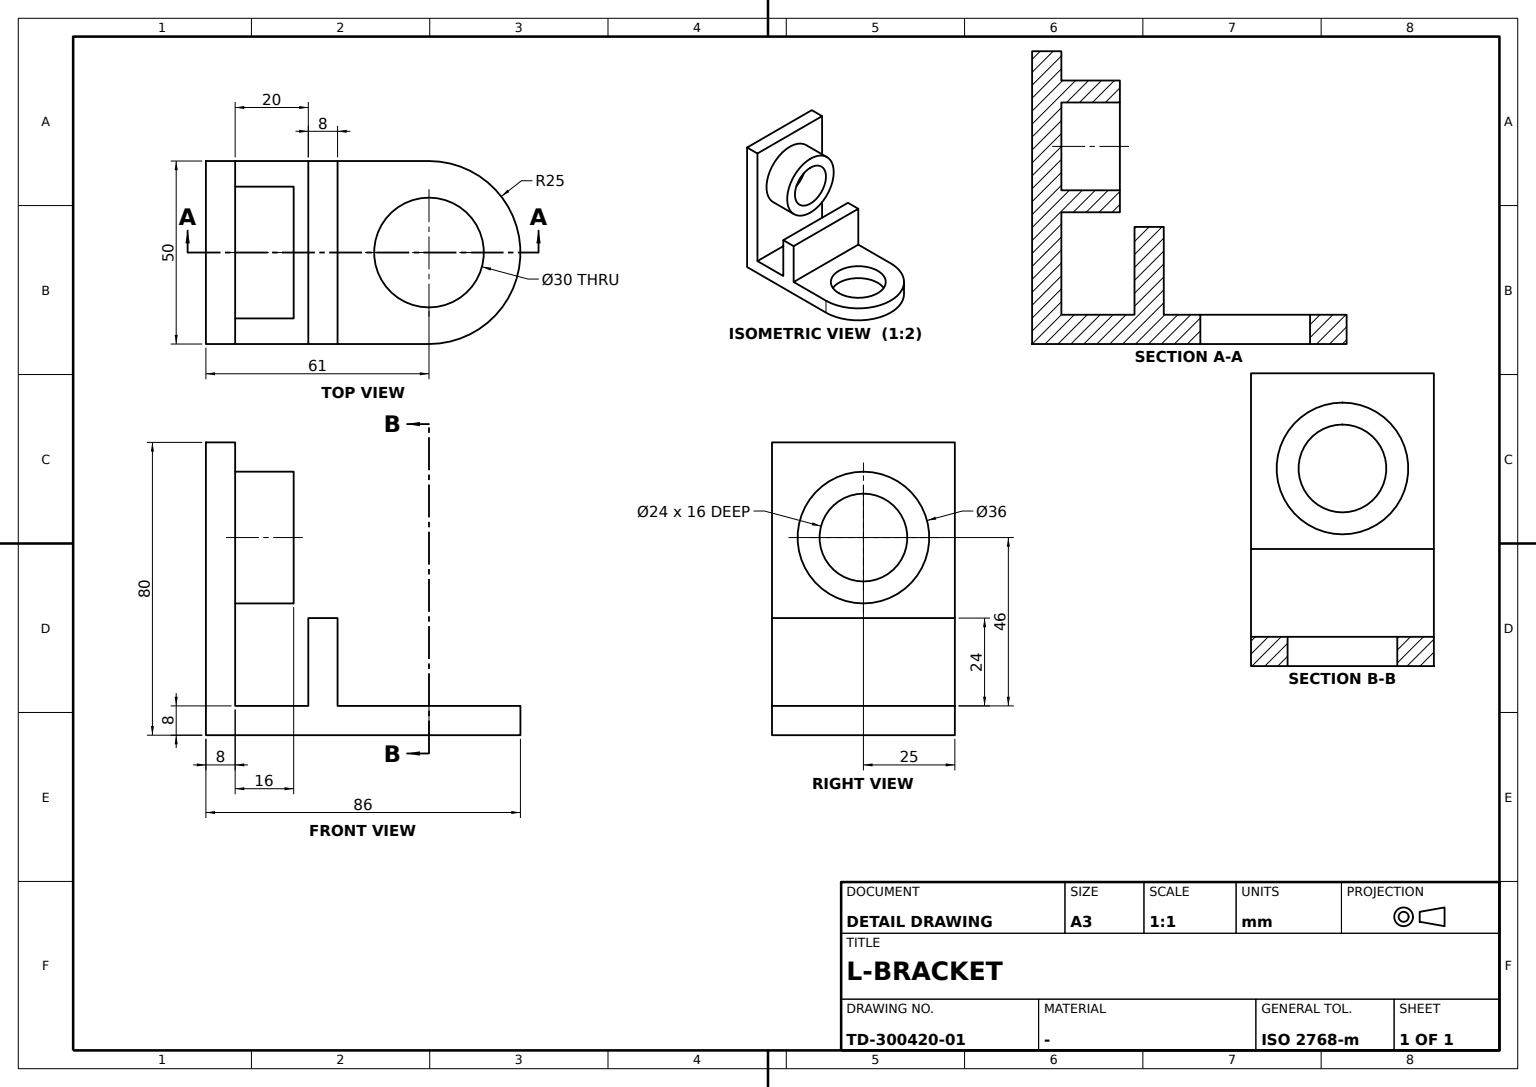
CATIA V5 part; units mm, degrees
sketch "Sketch1" plane through (0, 0, 0) normal (1, 0, 0) x (0, 1, 0)
  point P0 (0, 80)
  line L0 (0, 80) -> (0, 0)
  line L1 (0, 0) -> (36, 0)
  line L2 (36, 0) -> (36, 8)
  line L3 (28, 8) -> (8, 8)
  line L4 (8, 8) -> (8, 80)
  line L5 (8, 80) -> (0, 80)
  line L6 (28, 32) -> (36, 32)
  line L7 (36, 32) -> (36, 8)
  line L8 (28, 8) -> (28, 32)
  point P1 (28, 8)
  dimension "length L0" = 80
  dimension "length L5" = 8
  dimension "length L6" = 8
  dimension "length L3" = 20
  dimension "distance L3 x axis" = 8
  dimension "distance L6 P1" = 24
  constraint coincidence P0 y-axis
  constraint coincidence L7 L2
  constraint vertical L0 y-axis
  constraint vertical L2 y-axis
  constraint vertical L4 y-axis
  constraint vertical L7 y-axis
  constraint vertical L8 y-axis
  constraint horizontal L1 x-axis
  constraint horizontal L3 x-axis
  constraint horizontal L5 x-axis
  constraint horizontal L6 x-axis
extrude "Pad1" add sketch "Sketch1" along normal mid plane 50
sketch "Sketch2" plane through (0, 0, 0) normal (0, 0, 1) x (1, 0, 0)
  line L0 (-25, 61) -> (25, 61) construction
  line L1 (25, 61) -> (25, 36)
  line L2 (25, 36) -> (-25, 36)
  line L3 (-25, 36) -> (-25, 61)
  line L4 (-25, 36) -> (25, 36) construction
  arc A0 (25, 61) -> (-25, 61) centre (0, 61) ccw
  point P0 (0, 61)
  circle A1 centre (0, 61) radius 15
  dimension "length L0" = 50
  dimension "length L3" = 25
  dimension "distance L2 L4" = 0
  dimension "radius A1" = 15
  constraint horizontal L0 x-axis
  constraint horizontal L2 x-axis
  constraint vertical L1 y-axis
  constraint vertical L3 y-axis
  constraint symmetry L3 L1 y-axis
  constraint midpoint P0 L0
  constraint tangency A0 L1
extrude "Pad2" add sketch "Sketch2" along normal blind 8
sketch "Sketch3" plane through (0, 0, 0) normal (0, 1, 0) x (-1, 0, 0)
  circle A0 centre (0, 54) radius 18
  point P0 (0, 54)
  circle A1 centre (0, 54) radius 12
  line L0 (-25, 8) -> (25, 8) construction
  dimension "radius A1" = 12
  dimension "radius A0" = 18
  dimension "distance P0 L0" = 46
  constraint coincidence P0 y-axis
extrude "Pad3" add sketch "Sketch3" along normal blind 24
properties part number "6"
